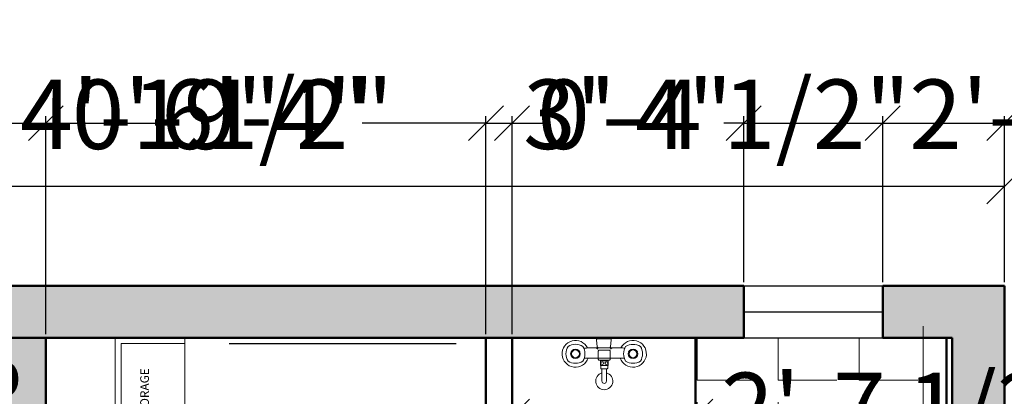
# Model space of a CAD drawing. Units: inches. Extents: x 2371 to 3019, y 129 to 700.
# Tile 13 of 14: x 2753 to 2923, y 612 to 677. Entities that reach past the tile are written whole.
import ezdxf

# ---------------------------------------------------------------- set-up
doc = ezdxf.new("R2010")
doc.units = ezdxf.units.IN
for name, color, linetype, lineweight in [('A-ANNO-DIMS', 2, 'Continuous', 18), ('A-AREA-IDEN', 7, 'Continuous', 25), ('A-FLOR-FIXT', 8, 'Continuous', 18), ('A-FLOR-PATT', 252, 'Continuous', 13), ('A-FURN', 8, 'Continuous', 18), ('A-GLAZ', 4, 'Continuous', 25), ('A-WALL', 7, 'Continuous', 50), ('A-WALL-PATT', 8, 'Continuous', 13)]:
    doc.layers.add(name, color=color, linetype=linetype, lineweight=lineweight)
doc.styles.get("Standard").update_dxf_attribs({"font": 'arial.ttf'})
doc.dimstyles.new('ISO-25', dxfattribs={"dimtxt": 12, "dimasz": 6, "dimexe": 1.25, "dimexo": 0.625, "dimtad": 0, "dimdec": 1, "dimlunit": 3, "dimtxsty": 'Standard', "dimblk": 'OBLIQUE', "dimblk1": 'ORIGIN2', "dimblk2": 'OBLIQUE', "dimcen": 2.5, "dimadec": 0, "dimazin": 0, "dimtfac": 1, "dimtdec": 1, "dimtmove": 0, "dimatfit": 3, "dimldrblk": 'OBLIQUE', "dimfxl": 1, "dimarcsym": 0})

# ---------------------------------------------------------------- blocks, each defined once
blk = doc.blocks.new('_Oblique')
at = {"color": 0, "linetype": 'ByBlock', "lineweight": -2}
blk.add_line((-0.5, -0.5), (0.5, 0.5), dxfattribs=at)
blk = doc.blocks.new('*D14')
at = {"layer": 'A-ANNO-DIMS', "color": 0, "lineweight": -2, "transparency": 16777216}
for p, q in [((2407.11, 631.6), (2407.11, 649.37)), ((2407.11, 648.12), (2643.63, 648.12)), ((2923.11, 648.12), (2686.58, 648.12)), ((2923.11, 631.6), (2923.11, 649.37))]:
    blk.add_line(p, q, dxfattribs=at)
at = {"layer": 'Defpoints', "color": 0, "lineweight": 25, "transparency": 16777216}
for p in [(2923.11, 648.12), (2407.11, 630.98), (2923.11, 630.98)]:
    blk.add_point(p, dxfattribs=at)
at = {"layer": 'A-ANNO-DIMS', "color": 0, "lineweight": -2, "transparency": 16777216, "xscale": 6, "yscale": 6, "zscale": 6, "rotation": 180}
blk.add_blockref('_Oblique', (2407.11, 648.12), dxfattribs=at)
at = {"layer": 'A-ANNO-DIMS', "color": 0, "lineweight": -2, "transparency": 16777216, "xscale": 6, "yscale": 6, "zscale": 6}
blk.add_blockref('_Oblique', (2923.11, 648.12), dxfattribs=at)
at = {"layer": 'A-ANNO-DIMS', "color": 0, "transparency": 16777216, "insert": (2665.11, 648.12), "char_height": 12, "width": 20.8486, "attachment_point": 5}
blk.add_mtext('43\'-0"', dxfattribs=at)
blk = doc.blocks.new('_Origin2')
at = {"color": 0, "linetype": 'ByBlock', "lineweight": -2}
blk.add_line((-0.5, 0), (-1, 0), dxfattribs=at)
for radius in [0.5, 0.25]:
    blk.add_circle((0, 0), radius, dxfattribs=at)
blk = doc.blocks.new('SHOWER-MIXER')
for points in [[(2508.84, 620.5, 0.281574), (2506.28, 620.5, 3.55146)], [(2511.46, 620.27), (2511.32, 620.45), (2511.19, 621.61, -0.472691), (2511.38, 621.8)], [(2513.47, 620.27), (2513.61, 620.45), (2513.75, 621.61, 0.472691), (2513.56, 621.8)], [(2516.23, 620.5, -0.281574), (2518.78, 620.5, -3.55146)], [(2506.28, 620.5, 0.281574), (2506.28, 617.95, 3.55146)], [(2508.84, 617.95, 0.281574), (2508.84, 620.5, 3.55146)], [(2508.98, 620.21, -0.00159), (2509.64, 620.23, 0.018232)], [(2509.64, 620.23, -0.004447), (2511.46, 620.27, -0.00338)], [(2511.46, 620.27, -0.000907), (2511.84, 620.27, -0.00338), (2513.23, 620.27, -0.000601), (2513.47, 620.27, 0.018232)], [(2511.5, 618.49), (2511.5, 619.7, -0.414214), (2511.66, 619.86), (2512.53, 619.86)], [(2513.56, 618.49), (2513.56, 619.7, 0.414214), (2513.4, 619.86), (2512.53, 619.86)], [(2513.47, 620.27, -0.004754), (2515.42, 620.24, 0.018232)], [(2515.42, 620.24, -0.00159), (2516.08, 620.22, 0.018232)], [(2516.23, 617.95, -0.281574), (2516.23, 620.5, -3.55146)], [(2518.78, 620.5, -0.281574), (2518.78, 617.95, -3.55146)], [(2506.28, 617.95, 0.281574), (2508.84, 617.95, 3.55146)], [(2511.5, 618.28), (2511.5, 618.49, -0.414214)], [(2511.86, 618.13), (2511.66, 618.13, -0.414214), (2511.5, 618.28)], [(2511.86, 618.13), (2511.86, 617.24, 0.414214), (2511.92, 617.18), (2511.93, 617.18)], [(2512.53, 618.13), (2511.86, 618.13, -0.414214)], [(2511.93, 617.18), (2511.93, 616.73, 0.414214), (2512.06, 616.6), (2512.09, 616.6), (2512.14, 616.6)], [(2512.53, 618.13), (2513.2, 618.13, 0.414214)], [(2513.13, 617.18), (2513.13, 616.73, -0.414214), (2513.01, 616.6), (2512.98, 616.6), (2512.92, 616.6)], [(2513.2, 618.13), (2513.2, 617.24, -0.414214), (2513.14, 617.18), (2513.13, 617.18)], [(2513.2, 618.13), (2513.4, 618.13, 0.414214), (2513.56, 618.28)], [(2513.56, 618.28), (2513.56, 618.49, 0.414214)], [(2518.78, 617.95, -0.281574), (2516.23, 617.95, -3.55146)], [(2512.14, 616.6), (2512.14, 615.94, 1)], [(2512.14, 615.94), (2512.14, 614.51, 1), (2512.92, 614.51), (2512.92, 615.94)]]:
    blk.add_lwpolyline(points, format="xyb")
for points in [[(2511.38, 621.8), (2512.47, 621.8)], [(2513.56, 621.8), (2512.47, 621.8)], [(2511.15, 620.27), (2511.42, 620.04)], [(2513.92, 620.27), (2513.64, 620.04)], [(2509.08, 618.49), (2509.75, 618.49)], [(2509.75, 618.49), (2511.5, 618.49)], [(2511.5, 618.49), (2513.56, 618.49)], [(2511.86, 618.01), (2512.53, 618.01)], [(2511.93, 617.18), (2512.53, 617.18)], [(2513.21, 618.01), (2512.53, 618.01)], [(2513.13, 617.18), (2512.53, 617.18)], [(2513.56, 618.49), (2515.31, 618.49)], [(2515.31, 618.49), (2515.98, 618.49)], [(2512.14, 616.6), (2512.53, 616.6)], [(2512.92, 616.6), (2512.53, 616.6)], [(2512.92, 615.94), (2512.92, 616.6)]]:
    blk.add_lwpolyline(points)
for centre, radius in [((2507.56, 619.22), 0.83), ((2507.56, 619.22), 0.674), ((2517.5, 619.22), 0.83), ((2517.5, 619.22), 0.674), ((2512.16, 617.6), 0.25), ((2512.9, 617.6), 0.25)]:
    blk.add_circle(centre, radius)
for centre, radius, start, end in [((2507.56, 619.22), 2.31, 25.9781, 341.5868), ((2517.5, 619.22), 2.31, 198.4132, 154.0219), ((2512.53, 614.51), 1.48, 105.2575, 74.7425)]:
    blk.add_arc(centre, radius, start, end)
blk = doc.blocks.new('*D30')
at = {"layer": 'A-ANNO-DIMS', "color": 0, "lineweight": -2, "transparency": 16777216}
for p, q in [((2505.18, 612.41), (2505.18, 609.58)), ((2519.88, 612.41), (2519.88, 609.58)), ((2505.18, 610.83), (2519.88, 610.83)), ((2519.88, 610.83), (2525.88, 610.83))]:
    blk.add_line(p, q, dxfattribs=at)
at = {"layer": 'Defpoints', "color": 0, "lineweight": 25, "transparency": 16777216}
for p in [(2505.18, 613.03), (2519.88, 613.03), (2519.88, 610.83)]:
    blk.add_point(p, dxfattribs=at)
at = {"layer": 'A-ANNO-DIMS', "color": 0, "lineweight": -2, "transparency": 16777216, "xscale": 6, "yscale": 6, "zscale": 6, "rotation": 180}
blk.add_blockref('_Oblique', (2505.18, 610.83), dxfattribs=at)
at = {"layer": 'A-ANNO-DIMS', "color": 0, "lineweight": -2, "transparency": 16777216, "xscale": 6, "yscale": 6, "zscale": 6}
blk.add_blockref('_Oblique', (2519.88, 610.83), dxfattribs=at)
at = {"layer": 'A-ANNO-DIMS', "color": 0, "transparency": 16777216, "insert": (2645.95, 610.83), "char_height": 12, "attachment_point": 5}
blk.add_mtext('SHOWER MIXER 1\'-2 1/2" TYP.', dxfattribs=at)
blk = doc.blocks.new('*D43')
at = {"layer": 'A-ANNO-DIMS', "color": 0, "lineweight": -2, "transparency": 16777216}
for p, q in [((2699.23, 631.6), (2699.23, 660.28)), ((2748.61, 622.6), (2748.61, 660.28)), ((2699.23, 659.03), (2748.61, 659.03)), ((2748.61, 659.03), (2754.61, 659.03))]:
    blk.add_line(p, q, dxfattribs=at)
at = {"layer": 'Defpoints', "color": 0, "lineweight": 25, "transparency": 16777216}
for p in [(2748.61, 659.03), (2699.23, 630.98), (2748.61, 621.98)]:
    blk.add_point(p, dxfattribs=at)
at = {"layer": 'A-ANNO-DIMS', "color": 0, "lineweight": -2, "transparency": 16777216, "xscale": 6, "yscale": 6, "zscale": 6, "rotation": 180}
blk.add_blockref('_Oblique', (2699.23, 659.03), dxfattribs=at)
at = {"layer": 'A-ANNO-DIMS', "color": 0, "lineweight": -2, "transparency": 16777216, "xscale": 6, "yscale": 6, "zscale": 6}
blk.add_blockref('_Oblique', (2748.61, 659.03), dxfattribs=at)
at = {"layer": 'A-ANNO-DIMS', "color": 0, "transparency": 16777216, "insert": (2785.4, 659.03), "char_height": 12, "attachment_point": 5}
blk.add_mtext('4\'-1 1/2"', dxfattribs=at)
blk = doc.blocks.new('*D44')
at = {"layer": 'A-ANNO-DIMS', "color": 0, "lineweight": -2, "transparency": 16777216}
for p, q in [((2748.61, 622.6), (2748.61, 660.28)), ((2757.61, 622.6), (2757.61, 660.28)), ((2748.61, 659.03), (2757.61, 659.03)), ((2757.61, 659.03), (2763.61, 659.03))]:
    blk.add_line(p, q, dxfattribs=at)
at = {"layer": 'Defpoints', "color": 0, "lineweight": 25, "transparency": 16777216}
for p in [(2757.61, 659.03), (2748.61, 621.98), (2757.61, 621.98)]:
    blk.add_point(p, dxfattribs=at)
at = {"layer": 'A-ANNO-DIMS', "color": 0, "lineweight": -2, "transparency": 16777216, "xscale": 6, "yscale": 6, "zscale": 6, "rotation": 180}
blk.add_blockref('_Oblique', (2748.61, 659.03), dxfattribs=at)
at = {"layer": 'A-ANNO-DIMS', "color": 0, "lineweight": -2, "transparency": 16777216, "xscale": 6, "yscale": 6, "zscale": 6}
blk.add_blockref('_Oblique', (2757.61, 659.03), dxfattribs=at)
at = {"layer": 'A-ANNO-DIMS', "color": 0, "transparency": 16777216, "insert": (2780.18, 659.03), "char_height": 12, "attachment_point": 5}
blk.add_mtext('0\'-9"', dxfattribs=at)
blk = doc.blocks.new('*D45')
at = {"layer": 'A-ANNO-DIMS', "color": 0, "lineweight": -2, "transparency": 16777216}
for p, q in [((2757.61, 622.6), (2757.61, 660.28)), ((2833.61, 622.6), (2833.61, 660.28)), ((2757.61, 659.03), (2779, 659.03)), ((2833.61, 659.03), (2812.21, 659.03))]:
    blk.add_line(p, q, dxfattribs=at)
at = {"layer": 'Defpoints', "color": 0, "lineweight": 25, "transparency": 16777216}
for p in [(2833.61, 659.03), (2757.61, 621.98), (2833.61, 621.98)]:
    blk.add_point(p, dxfattribs=at)
at = {"layer": 'A-ANNO-DIMS', "color": 0, "lineweight": -2, "transparency": 16777216, "xscale": 6, "yscale": 6, "zscale": 6, "rotation": 180}
blk.add_blockref('_Oblique', (2757.61, 659.03), dxfattribs=at)
at = {"layer": 'A-ANNO-DIMS', "color": 0, "lineweight": -2, "transparency": 16777216, "xscale": 6, "yscale": 6, "zscale": 6}
blk.add_blockref('_Oblique', (2833.61, 659.03), dxfattribs=at)
at = {"layer": 'A-ANNO-DIMS', "color": 0, "transparency": 16777216, "insert": (2795.61, 659.03), "char_height": 12, "attachment_point": 5}
blk.add_mtext('6\'-4"', dxfattribs=at)
blk = doc.blocks.new('*D46')
at = {"layer": 'A-ANNO-DIMS', "color": 0, "lineweight": -2, "transparency": 16777216}
for p, q in [((2833.61, 622.6), (2833.61, 660.28)), ((2838.11, 622.6), (2838.11, 660.28)), ((2833.61, 659.03), (2838.11, 659.03)), ((2838.11, 659.03), (2844.11, 659.03))]:
    blk.add_line(p, q, dxfattribs=at)
at = {"layer": 'Defpoints', "color": 0, "lineweight": 25, "transparency": 16777216}
for p in [(2838.11, 659.03), (2833.61, 621.98), (2838.11, 621.98)]:
    blk.add_point(p, dxfattribs=at)
at = {"layer": 'A-ANNO-DIMS', "color": 0, "lineweight": -2, "transparency": 16777216, "xscale": 6, "yscale": 6, "zscale": 6, "rotation": 180}
blk.add_blockref('_Oblique', (2833.61, 659.03), dxfattribs=at)
at = {"layer": 'A-ANNO-DIMS', "color": 0, "lineweight": -2, "transparency": 16777216, "xscale": 6, "yscale": 6, "zscale": 6}
blk.add_blockref('_Oblique', (2838.11, 659.03), dxfattribs=at)
at = {"layer": 'A-ANNO-DIMS', "color": 0, "transparency": 16777216, "insert": (2874.66, 659.03), "char_height": 12, "attachment_point": 5}
blk.add_mtext('0\'-4 1/2"', dxfattribs=at)
blk = doc.blocks.new('*D47')
at = {"layer": 'A-ANNO-DIMS', "color": 0, "lineweight": -2, "transparency": 16777216}
for p, q in [((2838.11, 622.6), (2838.11, 660.28)), ((2878.11, 631.6), (2878.11, 660.28)), ((2838.11, 659.03), (2841.53, 659.03)), ((2878.11, 659.03), (2874.68, 659.03))]:
    blk.add_line(p, q, dxfattribs=at)
at = {"layer": 'Defpoints', "color": 0, "lineweight": 25, "transparency": 16777216}
for p in [(2878.11, 659.03), (2878.11, 630.98), (2838.11, 621.98)]:
    blk.add_point(p, dxfattribs=at)
at = {"layer": 'A-ANNO-DIMS', "color": 0, "lineweight": -2, "transparency": 16777216, "xscale": 6, "yscale": 6, "zscale": 6, "rotation": 180}
blk.add_blockref('_Oblique', (2838.11, 659.03), dxfattribs=at)
at = {"layer": 'A-ANNO-DIMS', "color": 0, "lineweight": -2, "transparency": 16777216, "xscale": 6, "yscale": 6, "zscale": 6}
blk.add_blockref('_Oblique', (2878.11, 659.03), dxfattribs=at)
at = {"layer": 'A-ANNO-DIMS', "color": 0, "transparency": 16777216, "insert": (2858.11, 659.03), "char_height": 12, "attachment_point": 5}
blk.add_mtext('3\'-4"', dxfattribs=at)
blk = doc.blocks.new('*D48')
at = {"layer": 'A-ANNO-DIMS', "color": 0, "lineweight": -2, "transparency": 16777216}
for p, q in [((2878.11, 631.6), (2878.11, 660.28)), ((2902.11, 631.6), (2902.11, 660.28)), ((2878.11, 659.03), (2902.11, 659.03)), ((2902.11, 659.03), (2908.11, 659.03))]:
    blk.add_line(p, q, dxfattribs=at)
at = {"layer": 'Defpoints', "color": 0, "lineweight": 25, "transparency": 16777216}
for p in [(2902.11, 659.03), (2878.11, 630.98), (2902.11, 630.98)]:
    blk.add_point(p, dxfattribs=at)
at = {"layer": 'A-ANNO-DIMS', "color": 0, "lineweight": -2, "transparency": 16777216, "xscale": 6, "yscale": 6, "zscale": 6, "rotation": 180}
blk.add_blockref('_Oblique', (2878.11, 659.03), dxfattribs=at)
at = {"layer": 'A-ANNO-DIMS', "color": 0, "lineweight": -2, "transparency": 16777216, "xscale": 6, "yscale": 6, "zscale": 6}
blk.add_blockref('_Oblique', (2902.11, 659.03), dxfattribs=at)
at = {"layer": 'A-ANNO-DIMS', "color": 0, "transparency": 16777216, "insert": (2924.78, 659.03), "char_height": 12, "attachment_point": 5}
blk.add_mtext('2\'-0"', dxfattribs=at)
blk = doc.blocks.new('*D49')
at = {"layer": 'A-ANNO-DIMS', "color": 0, "lineweight": -2, "transparency": 16777216}
for p, q in [((2902.11, 631.6), (2902.11, 660.28)), ((2923.11, 631.6), (2923.11, 660.28)), ((2902.11, 659.03), (2923.11, 659.03)), ((2923.11, 659.03), (2929.11, 659.03))]:
    blk.add_line(p, q, dxfattribs=at)
at = {"layer": 'Defpoints', "color": 0, "lineweight": 25, "transparency": 16777216}
for p in [(2923.11, 659.03), (2902.11, 630.98), (2923.11, 630.98)]:
    blk.add_point(p, dxfattribs=at)
at = {"layer": 'A-ANNO-DIMS', "color": 0, "lineweight": -2, "transparency": 16777216, "xscale": 6, "yscale": 6, "zscale": 6, "rotation": 180}
blk.add_blockref('_Oblique', (2902.11, 659.03), dxfattribs=at)
at = {"layer": 'A-ANNO-DIMS', "color": 0, "lineweight": -2, "transparency": 16777216, "xscale": 6, "yscale": 6, "zscale": 6}
blk.add_blockref('_Oblique', (2923.11, 659.03), dxfattribs=at)
at = {"layer": 'A-ANNO-DIMS', "color": 0, "transparency": 16777216, "insert": (2945.11, 659.03), "char_height": 12, "attachment_point": 5}
blk.add_mtext('1\'-9"', dxfattribs=at)
blk = doc.blocks.new('*D77')
at = {"layer": 'A-ANNO-DIMS', "color": 0, "lineweight": -2, "transparency": 16777216}
for p, q in [((2838.11, 580.98), (2838.11, 609.66)), ((2869.78, 580.98), (2869.78, 609.66)), ((2838.11, 608.41), (2869.78, 608.41)), ((2869.78, 608.41), (2875.78, 608.41))]:
    blk.add_line(p, q, dxfattribs=at)
at = {"layer": 'Defpoints', "color": 0, "lineweight": 25, "transparency": 16777216}
for p in [(2869.78, 608.41), (2838.11, 580.36), (2869.78, 580.36)]:
    blk.add_point(p, dxfattribs=at)
at = {"layer": 'A-ANNO-DIMS', "color": 0, "lineweight": -2, "transparency": 16777216, "xscale": 6, "yscale": 6, "zscale": 6, "rotation": 180}
blk.add_blockref('_Oblique', (2838.11, 608.41), dxfattribs=at)
at = {"layer": 'A-ANNO-DIMS', "color": 0, "lineweight": -2, "transparency": 16777216, "xscale": 6, "yscale": 6, "zscale": 6}
blk.add_blockref('_Oblique', (2869.78, 608.41), dxfattribs=at)
at = {"layer": 'A-ANNO-DIMS', "color": 0, "transparency": 16777216, "insert": (2906.44, 608.41), "char_height": 12, "attachment_point": 5}
blk.add_mtext('2\'-7 1/2"', dxfattribs=at)

msp = doc.modelspace()

# ---------------------------------------------------------------- hatches: boundary and pattern name
at = {"layer": 'A-FLOR-PATT'}
h = msp.add_hatch(dxfattribs=at)
h.set_pattern_fill('_USER', color=256, scale=30, pattern_type=0)
h.set_pattern_definition([(0, (0, 0), (0, 30), [])])
h.paths.add_polyline_path([(2913.11, 498.98), (2827.61, 498.98), (2827.61, 531.98), (2832.11, 531.98), (2832.11, 537.98), (2833.61, 537.98), (2833.61, 605.98), (2818.35, 605.98, -1), (2796.86, 605.98), (2781.61, 605.98), (2781.61, 603.98), (2781.61, 533.98), (2757.61, 533.98), (2757.61, 531.98), (2797.61, 531.98), (2797.61, 522.98), (2757.61, 522.98), (2757.61, 516.98), (2754.59, 516.98), (2772.52, 485.76), (2771.01, 484.89), (2770.98, 484.93, -0.097552), (2757.61, 481.1), (2757.61, 422.48), (2837.61, 422.48), (2837.61, 362.48), (2757.61, 362.48), (2757.61, 303.98), (2835.86, 303.98, -0.09439), (2793.86, 311.98), (2793.86, 337.98), (2799.86, 337.98), (2799.86, 336.42), (2871.86, 336.42), (2871.86, 337.98), (2877.86, 337.98), (2877.86, 311.98, -0.09439), (2835.86, 303.98), (2913.11, 303.98), (2913.11, 383.18), (2904.11, 383.18), (2904.11, 419.18), (2913.11, 419.18)])
h.paths.add_polyline_path([(2788.88, 332.88), (2788.88, 308.88), (2764.88, 308.88), (2764.88, 332.88)], flags=16)
h.paths.add_polyline_path([(2788.4, 325.04, -1), (2774.4, 325.04, -1)], flags=0)
h.paths.add_polyline_path([(2781.4, 328.04), (2784.4, 325.04), (2781.4, 322.04), (2778.4, 325.04)], flags=0)
h.paths.add_polyline_path([(2782.4, 325.04, -1), (2780.4, 325.04, -1)], flags=0)
h.paths.add_polyline_path([(2748.61, 480.99), (2754.51, 480.98, 0.119303), (2770.98, 484.93), (2753.07, 516.1), (2754.59, 516.98), (2748.61, 516.98), (2748.61, 539.98), (2712.61, 539.98), (2665.11, 539.98, -0.09439), (2707.11, 531.98), (2707.11, 505.98), (2701.11, 505.98), (2701.11, 507.53), (2629.11, 507.53), (2629.11, 505.98), (2623.11, 505.98), (2623.11, 531.98, -0.09439), (2665.11, 539.98), (2581.61, 539.98), (2581.61, 522.98), (2581.61, 477.98, -0.131044), (2589.61, 507.98), (2615.61, 507.98), (2615.61, 501.98), (2614.05, 501.98), (2614.05, 453.98), (2615.61, 453.98), (2615.61, 447.98), (2589.61, 447.98, -0.131044), (2581.61, 477.98), (2581.61, 432.98), (2572.61, 432.98, 0.119303), (2556.14, 428.99), (2574.12, 397.85), (2572.61, 396.98), (2578.61, 396.98), (2581.61, 396.98), (2581.61, 390.98), (2748.61, 390.98)])
h.paths.add_polyline_path([(2683.1, 447.25), (2652.43, 447.25), (2652.43, 492.22), (2683.1, 492.22)], flags=16)
h.paths.add_polyline_path([(2682.1, 448.25), (2653.43, 448.25), (2653.43, 491.22), (2682.1, 491.22)], flags=0)
h.paths.add_polyline_path([(2613.58, 512.06), (2589.58, 512.06), (2589.58, 536.06), (2613.58, 536.06)], flags=16)
h.paths.add_polyline_path([(2599.1, 528.22, -1), (2613.1, 528.22, -1)], flags=0)
h.paths.add_polyline_path([(2609.1, 528.22), (2606.1, 525.22), (2603.1, 528.22), (2606.1, 531.22)], flags=0)
h.paths.add_polyline_path([(2607.1, 528.22, -1), (2605.1, 528.22, -1)], flags=0)
h.paths.add_polyline_path([(2581.61, 522.98), (2581.61, 621.98), (2572.61, 621.98), (2572.61, 522.98), (2572.61, 500.98), (2565.85, 500.98), (2565.85, 500.15), (2564.82, 500.15), (2561.16, 500.19), (2561.16, 500.17), (2560.13, 500.3), (2560.22, 500.98), (2556.38, 500.98), (2556.43, 500.22), (2555.4, 500.14), (2555.34, 500.98), (2551.07, 500.98), (2551.07, 500.15), (2550.04, 500.15), (2547.64, 500.19), (2547.64, 500.15), (2546.61, 500.15), (2541.79, 500.22), (2540.72, 500.13), (2540.65, 500.98), (2533.37, 500.98), (2533.37, 500.15), (2532.34, 500.15), (2529.13, 500.21), (2529.12, 500.13), (2528.09, 500.22), (2528.16, 500.98), (2523.23, 500.98), (2523.23, 500.15), (2522.2, 500.15), (2519.8, 500.21), (2519.8, 500.15), (2518.77, 500.15), (2514.45, 500.26), (2514.44, 500.14), (2513.41, 500.22), (2513.47, 500.98), (2509.62, 500.98), (2509.71, 500.3), (2508.69, 500.17), (2508.58, 500.98), (2505.03, 500.98), (2505.03, 500.15), (2503.99, 500.15), (2501.07, 500.29), (2501.07, 500.15), (2500.04, 500.15), (2496.44, 500.37), (2496.44, 500.15), (2495.4, 500.15), (2492.55, 500.41), (2492.18, 500.35), (2492.09, 500.98), (2486.11, 500.98), (2486.11, 524.98), (2486.11, 531.98), (2490.61, 531.98), (2490.61, 537.98), (2492.11, 537.98), (2492.11, 605.98), (2476.85, 605.98, -1), (2455.36, 605.98), (2440.11, 605.98), (2440.11, 533.98), (2416.11, 533.98), (2416.11, 605.98), (2416.11, 621.98), (2536.61, 621.98), (2536.61, 630.98), (2407.11, 630.98), (2407.11, 363.98), (2416.11, 363.98), (2416.11, 431.48), (2496.11, 431.48), (2496.11, 371.48), (2416.11, 371.48), (2416.11, 303.98), (2494.36, 303.98, -0.09439), (2452.36, 311.98), (2452.36, 337.98), (2458.36, 337.98), (2458.36, 336.42), (2530.36, 336.42), (2530.36, 337.98), (2536.36, 337.98), (2536.36, 311.98, -0.09439), (2494.36, 303.98), (2572.61, 303.98), (2572.61, 381.98), (2572.61, 396.98), (2554.61, 428.15), (2556.12, 429.03), (2556.14, 428.99, -0.119303), (2572.61, 432.98), (2578.61, 432.98), (2581.61, 432.98)])
h.paths.add_polyline_path([(2450.11, 500.98), (2444.5, 500.98), (2444.44, 500.14), (2443.41, 500.22), (2443.47, 500.98), (2439.62, 500.98), (2439.71, 500.3), (2438.69, 500.17), (2438.58, 500.98), (2435.02, 500.98), (2435.02, 500.15), (2433.99, 500.15), (2433.99, 500.98), (2431.07, 500.98), (2431.07, 500.15), (2430.04, 500.15), (2430.04, 500.98), (2426.43, 500.98), (2426.43, 500.15), (2425.4, 500.15), (2425.4, 500.98), (2423.13, 500.98), (2423.2, 500.5), (2422.18, 500.35), (2422.09, 500.98), (2416.11, 500.98), (2416.11, 524.98), (2416.11, 531.98), (2450.11, 531.98), (2450.11, 522.98)], flags=16)
h.paths.add_polyline_path([(2449.11, 501.98), (2417.11, 501.98), (2417.11, 522.98), (2417.11, 523.98), (2449.11, 523.98)], flags=0)
h.paths.add_polyline_path([(2420.7, 510.73), (2419.36, 520.07), (2420.38, 520.22), (2421.74, 510.73), (2425.4, 510.73), (2425.4, 520.07), (2426.43, 520.07), (2426.43, 510.73), (2430.04, 510.73), (2430.04, 520.07), (2431.07, 520.07), (2431.07, 510.73), (2433.99, 510.73), (2433.99, 520.07), (2435.02, 520.07), (2435.02, 510.73), (2437.35, 510.73), (2436.18, 519.93), (2437.2, 520.06), (2438.39, 510.73), (2444.17, 510.73), (2444.85, 520.08), (2445.88, 520.01), (2445.21, 510.73)], flags=0)
h.paths.add_polyline_path([(2446.94, 336.11), (2446.94, 312.11), (2422.94, 312.11), (2422.94, 336.11)], flags=16)
h.paths.add_polyline_path([(2446.46, 328.27, -1), (2432.46, 328.27, -1)], flags=0)
h.paths.add_polyline_path([(2439.46, 331.27), (2442.46, 328.27), (2439.46, 325.27), (2436.46, 328.27)], flags=0)
h.paths.add_polyline_path([(2440.46, 328.27, -1), (2438.46, 328.27, -1)], flags=0)
h.paths.add_polyline_path([(2816, 444.88), (2866.87, 444.88), (2866.87, 463.54), (2816, 463.54)], flags=24)
h.paths.add_polyline_path([(2794.21, 558.3), (2833.34, 558.3), (2833.34, 576.96), (2794.21, 576.96)], flags=24)
h.paths.add_polyline_path([(2651.69, 411.53), (2711.04, 411.53), (2711.04, 430.19), (2651.69, 430.19)], flags=24)
h.paths.add_polyline_path([(2494.09, 444.88), (2544.97, 444.88), (2544.97, 463.54), (2494.09, 463.54)], flags=24)
h.paths.add_polyline_path([(2444.55, 565.02), (2483.69, 565.02), (2483.69, 583.68), (2444.55, 583.68)], flags=24)
h = msp.add_hatch(dxfattribs=at)
h.set_pattern_fill('_USER', color=256, scale=30, angle=90, pattern_type=0)
h.set_pattern_definition([(90, (0, 0), (-30, 2e-15), [])])
h.paths.add_polyline_path([(2913.11, 498.98), (2827.61, 498.98), (2827.61, 531.98), (2832.11, 531.98), (2832.11, 537.98), (2833.61, 537.98), (2833.61, 605.98), (2818.35, 605.98, -1), (2796.86, 605.98), (2781.61, 605.98), (2781.61, 603.98), (2781.61, 533.98), (2757.61, 533.98), (2757.61, 531.98), (2797.61, 531.98), (2797.61, 522.98), (2757.61, 522.98), (2757.61, 516.98), (2754.59, 516.98), (2772.52, 485.76), (2771.01, 484.89), (2770.98, 484.93, -0.097552), (2757.61, 481.1), (2757.61, 422.48), (2837.61, 422.48), (2837.61, 362.48), (2757.61, 362.48), (2757.61, 303.98), (2835.86, 303.98, -0.09439), (2793.86, 311.98), (2793.86, 337.98), (2799.86, 337.98), (2799.86, 336.42), (2871.86, 336.42), (2871.86, 337.98), (2877.86, 337.98), (2877.86, 311.98, -0.09439), (2835.86, 303.98), (2913.11, 303.98), (2913.11, 383.18), (2904.11, 383.18), (2904.11, 419.18), (2913.11, 419.18)])
h.paths.add_polyline_path([(2788.88, 332.88), (2788.88, 308.88), (2764.88, 308.88), (2764.88, 332.88)], flags=16)
h.paths.add_polyline_path([(2788.4, 325.04, -1), (2774.4, 325.04, -1)], flags=0)
h.paths.add_polyline_path([(2781.4, 328.04), (2784.4, 325.04), (2781.4, 322.04), (2778.4, 325.04)], flags=0)
h.paths.add_polyline_path([(2782.4, 325.04, -1), (2780.4, 325.04, -1)], flags=0)
h.paths.add_polyline_path([(2748.61, 480.99), (2754.51, 480.98, 0.119303), (2770.98, 484.93), (2753.07, 516.1), (2754.59, 516.98), (2748.61, 516.98), (2748.61, 539.98), (2712.61, 539.98), (2665.11, 539.98, -0.09439), (2707.11, 531.98), (2707.11, 505.98), (2701.11, 505.98), (2701.11, 507.53), (2629.11, 507.53), (2629.11, 505.98), (2623.11, 505.98), (2623.11, 531.98, -0.09439), (2665.11, 539.98), (2581.61, 539.98), (2581.61, 522.98), (2581.61, 477.98, -0.131044), (2589.61, 507.98), (2615.61, 507.98), (2615.61, 501.98), (2614.05, 501.98), (2614.05, 453.98), (2615.61, 453.98), (2615.61, 447.98), (2589.61, 447.98, -0.131044), (2581.61, 477.98), (2581.61, 432.98), (2572.61, 432.98, 0.119303), (2556.14, 428.99), (2574.12, 397.85), (2572.61, 396.98), (2578.61, 396.98), (2581.61, 396.98), (2581.61, 390.98), (2748.61, 390.98)])
h.paths.add_polyline_path([(2683.1, 447.25), (2652.43, 447.25), (2652.43, 492.22), (2683.1, 492.22)], flags=16)
h.paths.add_polyline_path([(2682.1, 448.25), (2653.43, 448.25), (2653.43, 491.22), (2682.1, 491.22)], flags=0)
h.paths.add_polyline_path([(2613.58, 512.06), (2589.58, 512.06), (2589.58, 536.06), (2613.58, 536.06)], flags=16)
h.paths.add_polyline_path([(2599.1, 528.22, -1), (2613.1, 528.22, -1)], flags=0)
h.paths.add_polyline_path([(2609.1, 528.22), (2606.1, 525.22), (2603.1, 528.22), (2606.1, 531.22)], flags=0)
h.paths.add_polyline_path([(2607.1, 528.22, -1), (2605.1, 528.22, -1)], flags=0)
h.paths.add_polyline_path([(2581.61, 522.98), (2581.61, 621.98), (2572.61, 621.98), (2572.61, 522.98), (2572.61, 500.98), (2565.85, 500.98), (2565.85, 500.15), (2564.82, 500.15), (2561.16, 500.19), (2561.16, 500.17), (2560.13, 500.3), (2560.22, 500.98), (2556.38, 500.98), (2556.43, 500.22), (2555.4, 500.14), (2555.34, 500.98), (2551.07, 500.98), (2551.07, 500.15), (2550.04, 500.15), (2547.64, 500.19), (2547.64, 500.15), (2546.61, 500.15), (2541.79, 500.22), (2540.72, 500.13), (2540.65, 500.98), (2533.37, 500.98), (2533.37, 500.15), (2532.34, 500.15), (2529.13, 500.21), (2529.12, 500.13), (2528.09, 500.22), (2528.16, 500.98), (2523.23, 500.98), (2523.23, 500.15), (2522.2, 500.15), (2519.8, 500.21), (2519.8, 500.15), (2518.77, 500.15), (2514.45, 500.26), (2514.44, 500.14), (2513.41, 500.22), (2513.47, 500.98), (2509.62, 500.98), (2509.71, 500.3), (2508.69, 500.17), (2508.58, 500.98), (2505.03, 500.98), (2505.03, 500.15), (2503.99, 500.15), (2501.07, 500.29), (2501.07, 500.15), (2500.04, 500.15), (2496.44, 500.37), (2496.44, 500.15), (2495.4, 500.15), (2492.55, 500.41), (2492.18, 500.35), (2492.09, 500.98), (2486.11, 500.98), (2486.11, 524.98), (2486.11, 531.98), (2490.61, 531.98), (2490.61, 537.98), (2492.11, 537.98), (2492.11, 605.98), (2476.85, 605.98, -1), (2455.36, 605.98), (2440.11, 605.98), (2440.11, 533.98), (2416.11, 533.98), (2416.11, 605.98), (2416.11, 621.98), (2536.61, 621.98), (2536.61, 630.98), (2407.11, 630.98), (2407.11, 363.98), (2416.11, 363.98), (2416.11, 431.48), (2496.11, 431.48), (2496.11, 371.48), (2416.11, 371.48), (2416.11, 303.98), (2494.36, 303.98, -0.09439), (2452.36, 311.98), (2452.36, 337.98), (2458.36, 337.98), (2458.36, 336.42), (2530.36, 336.42), (2530.36, 337.98), (2536.36, 337.98), (2536.36, 311.98, -0.09439), (2494.36, 303.98), (2572.61, 303.98), (2572.61, 381.98), (2572.61, 396.98), (2554.61, 428.15), (2556.12, 429.03), (2556.14, 428.99, -0.119303), (2572.61, 432.98), (2578.61, 432.98), (2581.61, 432.98)])
h.paths.add_polyline_path([(2450.11, 500.98), (2444.5, 500.98), (2444.44, 500.14), (2443.41, 500.22), (2443.47, 500.98), (2439.62, 500.98), (2439.71, 500.3), (2438.69, 500.17), (2438.58, 500.98), (2435.02, 500.98), (2435.02, 500.15), (2433.99, 500.15), (2433.99, 500.98), (2431.07, 500.98), (2431.07, 500.15), (2430.04, 500.15), (2430.04, 500.98), (2426.43, 500.98), (2426.43, 500.15), (2425.4, 500.15), (2425.4, 500.98), (2423.13, 500.98), (2423.2, 500.5), (2422.18, 500.35), (2422.09, 500.98), (2416.11, 500.98), (2416.11, 524.98), (2416.11, 531.98), (2450.11, 531.98), (2450.11, 522.98)], flags=16)
h.paths.add_polyline_path([(2449.11, 501.98), (2417.11, 501.98), (2417.11, 522.98), (2417.11, 523.98), (2449.11, 523.98)], flags=0)
h.paths.add_polyline_path([(2420.7, 510.73), (2419.36, 520.07), (2420.38, 520.22), (2421.74, 510.73), (2425.4, 510.73), (2425.4, 520.07), (2426.43, 520.07), (2426.43, 510.73), (2430.04, 510.73), (2430.04, 520.07), (2431.07, 520.07), (2431.07, 510.73), (2433.99, 510.73), (2433.99, 520.07), (2435.02, 520.07), (2435.02, 510.73), (2437.35, 510.73), (2436.18, 519.93), (2437.2, 520.06), (2438.39, 510.73), (2444.17, 510.73), (2444.85, 520.08), (2445.88, 520.01), (2445.21, 510.73)], flags=0)
h.paths.add_polyline_path([(2446.94, 336.11), (2446.94, 312.11), (2422.94, 312.11), (2422.94, 336.11)], flags=16)
h.paths.add_polyline_path([(2446.46, 328.27, -1), (2432.46, 328.27, -1)], flags=0)
h.paths.add_polyline_path([(2439.46, 331.27), (2442.46, 328.27), (2439.46, 325.27), (2436.46, 328.27)], flags=0)
h.paths.add_polyline_path([(2440.46, 328.27, -1), (2438.46, 328.27, -1)], flags=0)
h.paths.add_polyline_path([(2816, 444.88), (2866.87, 444.88), (2866.87, 463.54), (2816, 463.54)], flags=24)
h.paths.add_polyline_path([(2794.21, 558.3), (2833.34, 558.3), (2833.34, 576.96), (2794.21, 576.96)], flags=24)
h.paths.add_polyline_path([(2651.69, 411.53), (2711.04, 411.53), (2711.04, 430.19), (2651.69, 430.19)], flags=24)
h.paths.add_polyline_path([(2494.09, 444.88), (2544.97, 444.88), (2544.97, 463.54), (2494.09, 463.54)], flags=24)
h.paths.add_polyline_path([(2444.55, 565.02), (2483.69, 565.02), (2483.69, 583.68), (2444.55, 583.68)], flags=24)
h = msp.add_hatch(dxfattribs=at)
h.set_pattern_fill('ANGLE', color=256, scale=2)
h.set_pattern_definition([(0, (341.5, 0), (0, 13.97), [10.16, -3.81]), (90, (341.5, 0), (-13.97, 9e-16), [10.16, -3.81])])
h.paths.add_polyline_path([(2909.11, 621.98), (2902.11, 621.98), (2878.11, 621.98), (2869.78, 621.98), (2869.78, 580.36), (2838.11, 580.36), (2838.11, 569.98), (2833.61, 569.98), (2833.61, 537.98), (2838.11, 537.98), (2838.11, 531.98), (2883.14, 531.98), (2883.14, 563.44), (2909.11, 563.44)])
h.paths.add_polyline_path([(2877.58, 595.53, -0.215004), (2877.58, 598.82, -0.48008), (2895.11, 601.18), (2895.11, 593.18, -0.48008)], flags=16)
h.paths.add_polyline_path([(2902.11, 588.68), (2902.11, 605.68, -0.5), (2903.11, 606.68), (2907.11, 606.68, -0.5), (2908.11, 605.68), (2908.11, 588.68, -0.5), (2907.11, 587.68), (2903.11, 587.68, -0.5)], flags=16)
at = {"layer": 'A-WALL-PATT'}
h = msp.add_hatch(color=256, dxfattribs=at)
h.dxf.hatch_style = 1
h.paths.add_polyline_path([(2536.61, 630.98), (2407.11, 630.98), (2407.11, 363.98), (2416.11, 363.98), (2416.11, 498.98), (2416.11, 522.98), (2416.11, 531.98), (2416.11, 603.98), (2416.11, 621.98), (2536.61, 621.98)])
h.paths.add_polyline_path([(2630.98, 630.98), (2560.61, 630.98), (2560.61, 621.98), (2630.98, 621.98)])
h.paths.add_polyline_path([(2878.11, 630.98), (2699.23, 630.98), (2699.23, 621.98), (2878.11, 621.98)])
h.paths.add_polyline_path([(2496.61, 621.98), (2492.11, 621.98), (2492.11, 569.98), (2496.61, 569.98)], flags=17)
h.paths.add_polyline_path([(2581.61, 621.98), (2572.61, 621.98), (2572.61, 522.98), (2572.61, 498.98), (2572.61, 432.98), (2578.61, 432.98), (2581.61, 432.98), (2581.61, 522.98)])
h.paths.add_polyline_path([(2572.61, 531.98), (2486.11, 531.98), (2486.11, 522.98), (2572.61, 522.98)])
h.paths.add_polyline_path([(2450.11, 531.98), (2440.11, 531.98), (2416.11, 531.98), (2416.11, 522.98), (2450.11, 522.98)], flags=17)
h.paths.add_polyline_path([(2416.11, 315.98), (2407.11, 315.98), (2407.11, 294.98), (2458.11, 294.98), (2458.11, 303.98), (2416.11, 303.98)])
h.paths.add_polyline_path([(2757.61, 303.98), (2530.61, 303.98), (2530.61, 294.98), (2757.61, 294.98)])
h.paths.add_polyline_path([(2581.61, 381.98), (2605.61, 381.98), (2617.61, 381.98), (2617.61, 390.98), (2581.61, 390.98), (2581.61, 396.98), (2572.61, 396.98), (2572.61, 381.98), (2572.61, 303.98), (2581.61, 303.98)])
h.paths.add_polyline_path([(2757.61, 480.98), (2748.61, 480.98), (2748.61, 381.98), (2748.61, 303.98), (2757.61, 303.98), (2757.61, 381.98), (2757.61, 422.48)])
h.paths.add_polyline_path([(2797.61, 531.98), (2757.61, 531.98), (2757.61, 603.98), (2757.61, 621.98), (2748.61, 621.98), (2748.61, 516.99), (2754.59, 516.98), (2757.61, 516.98), (2757.61, 522.98), (2797.61, 522.98)])
h.paths.add_polyline_path([(2913.11, 531.98), (2827.61, 531.98), (2827.61, 522.98), (2913.11, 522.98)])
h.paths.add_polyline_path([(2923.11, 630.98), (2902.11, 630.98), (2902.11, 621.98), (2914.11, 621.98), (2914.11, 363.98), (2923.11, 363.98)])
h.paths.add_polyline_path([(2923.11, 315.98), (2914.11, 315.98), (2914.11, 303.98), (2866.11, 303.98), (2866.11, 294.98), (2923.11, 294.98)])
h.paths.add_polyline_path([(2793.61, 303.98), (2757.61, 303.98), (2757.61, 294.98), (2793.61, 294.98)])

# ---------------------------------------------------------------- linework, layer by layer
at = {"layer": 'A-FURN'}
for p, q in [((2909.11, 565.44), (2909.11, 623.98)), ((2769.61, 605.98), (2769.61, 621.98)), ((2781.61, 620.98), (2770.61, 620.98)), ((2770.61, 605.98), (2770.61, 620.98)), ((2781.61, 603.98), (2781.61, 621.98))]:
    msp.add_line(p, q, dxfattribs=at)
for points in [[(2852.88, 621.8, -0.080845), (2853.97, 621.98, -0.039297)], [(2855.06, 621.8, 0.080845), (2853.97, 621.98, 0.039297)]]:
    msp.add_lwpolyline(points, format="xyb", dxfattribs=at)
at = {"layer": 'A-GLAZ', "ltscale": 0.5}
for p, q in [((2878.11, 630.98), (2902.11, 630.98)), ((2878.11, 626.48), (2902.11, 626.48)), ((2878.11, 621.98), (2902.11, 621.98))]:
    msp.add_line(p, q, dxfattribs=at)
at = {"layer": 'A-GLAZ'}
msp.add_line((2789.29, 620.98), (2828.44, 620.98), dxfattribs=at)
at = {"layer": 'A-WALL'}
for p, q in [((2878.11, 630.98), (2560.61, 630.98)), ((2878.11, 621.98), (2878.11, 630.98)), ((2923.11, 630.98), (2902.11, 630.98)), ((2902.11, 621.98), (2902.11, 630.98)), ((2923.11, 294.98), (2923.11, 630.98)), ((2878.11, 621.98), (2560.61, 621.98)), ((2757.61, 531.98), (2757.61, 621.98)), ((2833.61, 537.98), (2833.61, 621.98)), ((2838.11, 569.98), (2838.11, 621.98)), ((2869.78, 621.98), (2869.78, 580.36)), ((2914.11, 621.98), (2902.11, 621.98)), ((2913.11, 522.98), (2913.11, 621.98)), ((2914.11, 303.98), (2914.11, 621.98))]:
    msp.add_line(p, q, dxfattribs=at)

# ---------------------------------------------------------------- block references
at = {"layer": 'A-FLOR-FIXT'}
msp.add_blockref('SHOWER-MIXER', (341.5, 0), dxfattribs=at)

# ---------------------------------------------------------------- texts
at = {"layer": 'A-AREA-IDEN', "insert": (2773.92, 607.61), "char_height": 1.5, "attachment_point": 1, "rotation": 90}
msp.add_mtext_dynamic_manual_height_columns('STORAGE', width=1.7945, gutter_width=12.5, heights=[0], dxfattribs=at)

# ---------------------------------------------------------------- dimensions: what is measured, and where the dimension line sits
at = {"layer": 'A-ANNO-DIMS'}
for base, p1, p2, picture, middle in [((2748.61, 659.03), (2699.23, 630.98), (2748.61, 621.98), '*D43', (2785.4, 659.03)), ((2838.11, 659.03), (2833.61, 621.98), (2838.11, 621.98), '*D46', (2874.66, 659.03)), ((2757.61, 659.03), (2748.61, 621.98), (2757.61, 621.98), '*D44', (2780.18, 659.03)), ((2833.61, 659.03), (2757.61, 621.98), (2833.61, 621.98), '*D45', (2795.61, 659.03)), ((2878.11, 659.03), (2838.11, 621.98), (2878.11, 630.98), '*D47', (2858.11, 659.03)), ((2902.11, 659.03), (2878.11, 630.98), (2902.11, 630.98), '*D48', (2924.78, 659.03)), ((2923.11, 659.03), (2902.11, 630.98), (2923.11, 630.98), '*D49', (2945.11, 659.03))]:
    dim = msp.add_linear_dim(base=base, p1=p1, p2=p2, dimstyle='ISO-25', override={"dimdec": 1, "dimlfac": 1, "dimrnd": 0, "dimzin": 1, "dimdsep": 46, "dimlunit": 4, "dimfrac": 2}, dxfattribs=at)
    dim.commit()
    dim.dimension.update_dxf_attribs({"geometry": picture, "text_midpoint": middle})
for base, p1, p2, text, override, picture, middle in [((2519.88, 610.83), (2505.18, 613.03), (2519.88, 613.03), 'SHOWER MIXER <> TYP.', {"dimdec": 1, "dimrnd": 0, "dimzin": 1, "dimlunit": 4, "dimfrac": 2}, '*D30', (2645.95, 610.83)), ((2923.11, 648.12), (2407.11, 630.98), (2923.11, 630.98), '43\'-0"', {"dimclrd": 0, "dimclre": 0, "dimclrt": 0}, '*D14', (2665.11, 648.12))]:
    dim = msp.add_linear_dim(base=base, p1=p1, p2=p2, text=text, dimstyle='ISO-25', override=override, dxfattribs=at)
    dim.commit()
    dim.dimension.update_dxf_attribs({"geometry": picture, "text_midpoint": middle})
dim = msp.add_linear_dim(base=(2869.78, 608.41), p1=(2838.11, 580.36), p2=(2869.78, 580.36), angle=0, dimstyle='ISO-25', override={"dimdec": 1, "dimlfac": 1, "dimrnd": 0, "dimzin": 1, "dimdsep": 46, "dimlunit": 4, "dimfrac": 2}, dxfattribs=at)
dim.commit()
dim.dimension.update_dxf_attribs({"geometry": '*D77', "text_midpoint": (2906.44, 608.41)})

doc.saveas('drawing.dxf')
